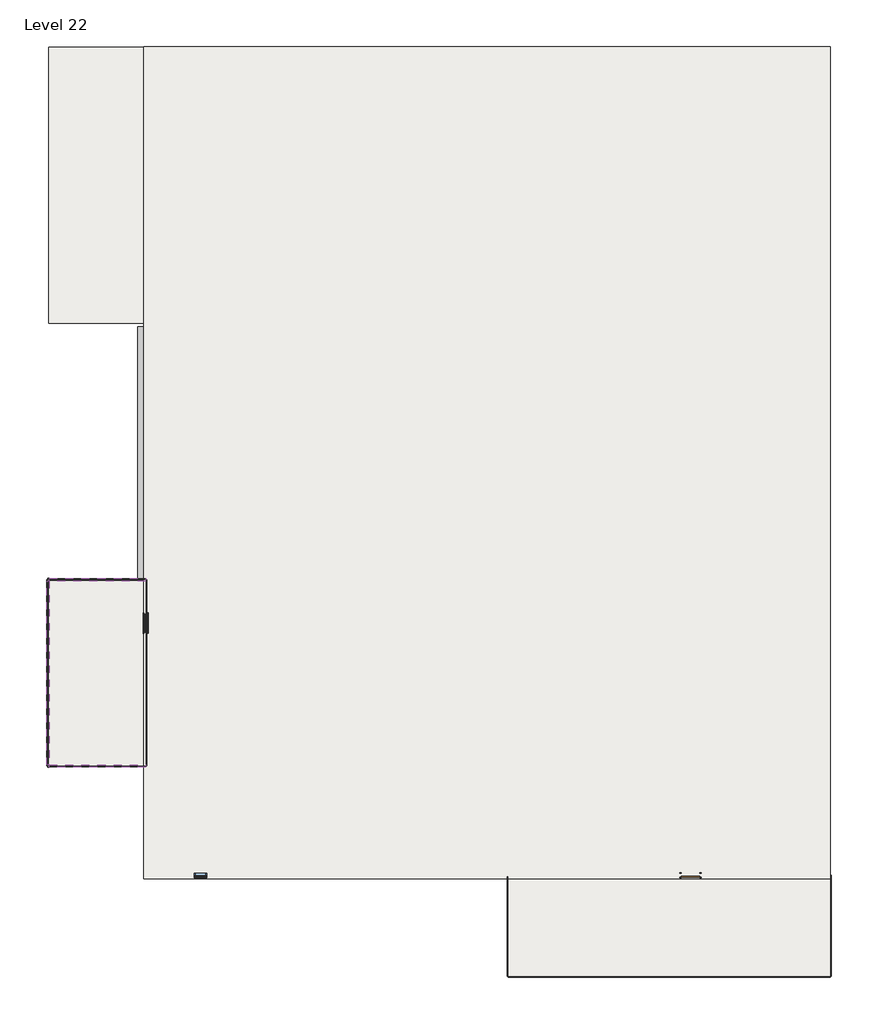
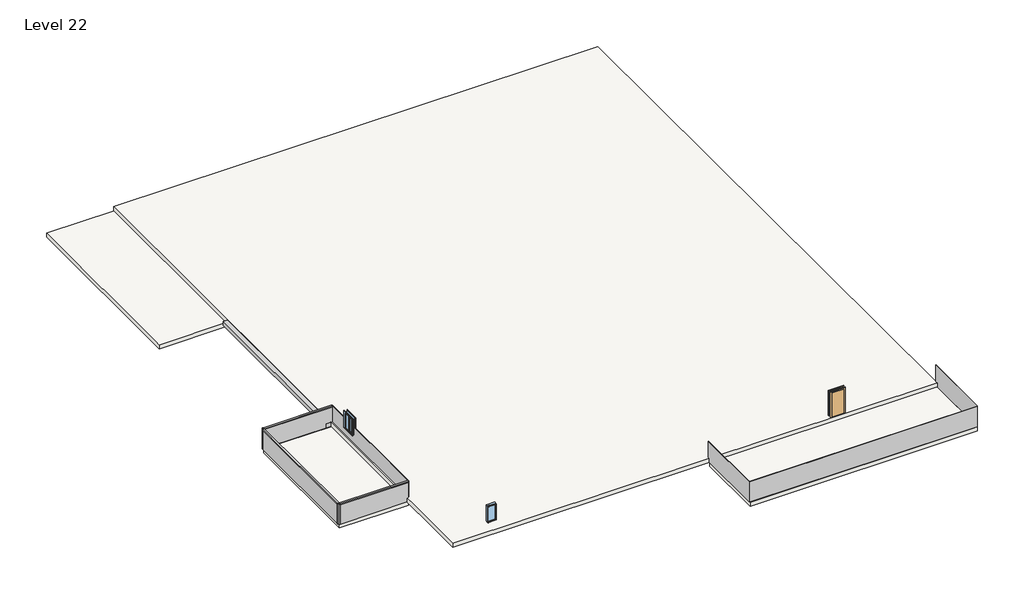
# One storey: 7 members, 7 plates, 4 slabs, 2 windows, 1 door, 1 proxy.
"""IFC4 building model written with IfcOpenShell, lengths in millimetres."""

from ifc_helpers import new_model, si_unit, frame, origin, place, context, project, spatial, polyline, outline, extrude, transform, mapped, element, save
from components import generic_models_7_generic_models_7_7f11944a, door_719f80de, member_4491d118, member_e63cd10b, member_1c0fec03, system_panel_glazed_dbf8c7ac, system_panel_glazed_9f3cc7a8, system_panel_glazed_aa9a1819, system_panel_glazed_da9a879b, system_panel_glazed_ba9ccfd0, system_panel_glazed_4de2f835, window_78885257, window_54100e87

model = new_model("IFC4")

# Units and contexts
model_context = context("Model", 3, world=origin())
ifc_project = project(units=[si_unit("LENGTHUNIT", "METRE", prefix="MILLI")], contexts=[model_context])

# Site, building, storey
site = spatial("IfcSite", under=ifc_project)
building = spatial("IfcBuilding", under=site)
storey = spatial("IfcBuildingStorey", under=building, Name="Level 22", Elevation=36271.2)

# Proxy
placement = place(None, origin())
generic_models_7_generic_models_7_shape = generic_models_7_generic_models_7_7f11944a(model_context)
element("IfcBuildingElementProxy", 1, Name="Generic Models 7 : Generic Models 7", ObjectType="Generic Models 7 : Generic Models 7", at=placement, inside=storey, context=model_context, shape_type="MappedRepresentation", body=[
    mapped(generic_models_7_generic_models_7_shape, transform((0.0, 0.0, 0.0), x_axis=(1.0, 0.0, 0.0), y_axis=(0.0, 1.0, 0.0), z_axis=(0.0, 0.0, 1.0))),
])

# Door
door_shape = door_719f80de(model_context)
element("IfcDoor", 2, ObjectType="Single-Flush : 36\" x 84\"", at=placement, inside=storey, context=model_context, shape_type="MappedRepresentation", body=[
    mapped(door_shape, transform((12155.361926, -20744.1985361, 36271.2), x_axis=(1.0, 0.0, 0.0), y_axis=(0.0, 1.0, 0.0), z_axis=(0.0, 0.0, 1.0))),
])

# Members
member_shape = member_4491d118(model_context)
element("IfcMember", 3, ObjectType="Rectangular Mullion : 2.5\" x 5\" rectangular", at=placement, inside=storey, context=model_context, shape_type="MappedRepresentation", body=[
    mapped(member_shape, transform((-20096.288074, -15263.2213044, 36271.2), x_axis=(-1.0, 0.0, 0.0), y_axis=(0.0, 1.0, 0.0), z_axis=(0.0, 0.0, -1.0))),
])
element("IfcMember", 4, ObjectType="Rectangular Mullion : 2.5\" x 5\" rectangular", at=placement, inside=storey, context=model_context, shape_type="MappedRepresentation", body=[
    mapped(member_shape, transform((-20096.288074, -5922.3713044, 36271.2), x_axis=(0.0, 1.0, 0.0), y_axis=(1.0, 0.0, 0.0), z_axis=(0.0, 0.0, -1.0))),
])
element("IfcMember", 5, ObjectType="Rectangular Mullion : 2.5\" x 5\" rectangular", at=placement, inside=storey, context=model_context, shape_type="MappedRepresentation", body=[
    mapped(member_shape, transform((-20096.288074, -15263.2213044, 37795.2), x_axis=(0.0, -1.0, 0.0), y_axis=(1.0, 0.0, 0.0), z_axis=(0.0, 0.0, 1.0))),
])
element("IfcMember", 6, ObjectType="Rectangular Mullion : 2.5\" x 5\" rectangular", at=placement, inside=storey, context=model_context, shape_type="MappedRepresentation", body=[
    mapped(member_shape, transform((-20096.288074, -5922.3713044, 37795.2), x_axis=(-1.0, 0.0, 0.0), y_axis=(0.0, -1.0, 0.0), z_axis=(0.0, 0.0, 1.0))),
])
member_2_shape = member_e63cd10b(model_context)
element("IfcMember", 7, ObjectType="Rectangular Mullion : 2.5\" x 5\" rectangular", at=placement, inside=storey, context=model_context, shape_type="MappedRepresentation", body=[
    mapped(member_2_shape, transform((-15175.038074, -5922.3713044, 37795.2), x_axis=(0.0, 0.0, 1.0), y_axis=(0.0, -1.0, 0.0), z_axis=(1.0, 0.0, 0.0))),
])
element("IfcMember", 8, ObjectType="Rectangular Mullion : 2.5\" x 5\" rectangular", at=placement, inside=storey, context=model_context, shape_type="MappedRepresentation", body=[
    mapped(member_2_shape, transform((-20032.788074, -15263.2213044, 37795.2), x_axis=(0.0, 0.0, 1.0), y_axis=(0.0, 1.0, 0.0), z_axis=(-1.0, 0.0, 0.0))),
])
member_3_shape = member_1c0fec03(model_context)
element("IfcMember", 9, ObjectType="Rectangular Mullion : 2.5\" x 5\" rectangular", at=placement, inside=storey, context=model_context, shape_type="MappedRepresentation", body=[
    mapped(member_3_shape, transform((-20096.288074, -5985.8713044, 37795.2), x_axis=(0.0, 0.0, 1.0), y_axis=(1.0, 0.0, 0.0), z_axis=(0.0, 1.0, 0.0))),
])

# Plates
system_panel_glazed_shape = system_panel_glazed_dbf8c7ac(model_context)
element("IfcPlate", 10, ObjectType="System Panel : Glazed", at=placement, inside=storey, context=model_context, shape_type="MappedRepresentation", body=[
    mapped(system_panel_glazed_shape, transform((11088.561926, -25828.3670305, 36271.2), x_axis=(-1.0, 0.0, 0.0), y_axis=(0.0, -1.0, 0.0), z_axis=(0.0, 0.0, 1.0))),
])
system_panel_glazed_2_shape = system_panel_glazed_9f3cc7a8(model_context)
element("IfcPlate", 11, ObjectType="System Panel : Glazed", at=placement, inside=storey, context=model_context, shape_type="MappedRepresentation", body=[
    mapped(system_panel_glazed_2_shape, transform((19165.761926, -23286.2827833, 36271.2), x_axis=(0.0, -1.0, 0.0), y_axis=(1.0, 0.0, 0.0), z_axis=(0.0, 0.0, 1.0))),
])
system_panel_glazed_3_shape = system_panel_glazed_aa9a1819(model_context)
element("IfcPlate", 12, ObjectType="System Panel : Glazed", at=placement, inside=storey, context=model_context, shape_type="MappedRepresentation", body=[
    mapped(system_panel_glazed_3_shape, transform((3011.361926, -23326.2903055, 36271.2), x_axis=(0.0, 1.0, 0.0), y_axis=(-1.0, 0.0, 0.0), z_axis=(0.0, 0.0, 1.0))),
])
system_panel_glazed_4_shape = system_panel_glazed_da9a879b(model_context)
element("IfcPlate", 13, ObjectType="System Panel : Glazed", at=placement, inside=storey, context=model_context, shape_type="MappedRepresentation", body=[
    mapped(system_panel_glazed_4_shape, transform((-15175.038074, -10592.7963044, 36271.2), x_axis=(0.0, -1.0, 0.0), y_axis=(1.0, 0.0, 0.0), z_axis=(0.0, 0.0, 1.0))),
])
system_panel_glazed_5_shape = system_panel_glazed_ba9ccfd0(model_context)
element("IfcPlate", 14, ObjectType="System Panel : Glazed", at=placement, inside=storey, context=model_context, shape_type="MappedRepresentation", body=[
    mapped(system_panel_glazed_5_shape, transform((-17603.913074, -5922.3713044, 36271.2), x_axis=(1.0, 0.0, 0.0), y_axis=(0.0, 1.0, 0.0), z_axis=(0.0, 0.0, 1.0))),
])
element("IfcPlate", 15, ObjectType="System Panel : Glazed", at=placement, inside=storey, context=model_context, shape_type="MappedRepresentation", body=[
    mapped(system_panel_glazed_5_shape, transform((-17603.913074, -15263.2213044, 36271.2), x_axis=(-1.0, 0.0, 0.0), y_axis=(0.0, -1.0, 0.0), z_axis=(0.0, 0.0, 1.0))),
])
system_panel_glazed_6_shape = system_panel_glazed_4de2f835(model_context)
element("IfcPlate", 16, ObjectType="System Panel : Glazed", at=placement, inside=storey, context=model_context, shape_type="MappedRepresentation", body=[
    mapped(system_panel_glazed_6_shape, transform((-20096.288074, -10592.7963044, 36271.2), x_axis=(0.0, 1.0, 0.0), y_axis=(-1.0, 0.0, 0.0), z_axis=(0.0, 0.0, 1.0))),
])

# Slabs
element("IfcSlab", 17, ObjectType="Generic - 12\"", at=placement, inside=storey, context=model_context, shape_type="SweptSolid", body=[
    extrude(outline(polyline([(19165.761926, 20833.4253594), (19165.761926, -20924.1746406), (-15276.638074, -20924.1746406), (-15276.638074, 20833.4253594), (19165.761926, 20833.4253594)])), frame((0.0, 0.0, 36258.4195447), z_axis=(0.0, 0.0, 1.0), x_axis=(1.0, 0.0, 0.0)), (0.0, 0.0, 1.0), 304.8),
])
element("IfcSlab", 18, ObjectType="Generic - 12\"", at=placement, inside=storey, context=model_context, shape_type="SweptSolid", body=[
    extrude(outline(polyline([(19165.761926, -20914.1789604), (19165.761926, -25879.1670305), (3011.361926, -25879.1670305), (3011.361926, -20914.1789604), (19165.761926, -20914.1789604)])), frame((0.0, 0.0, 35966.4), z_axis=(0.0, 0.0, 1.0), x_axis=(1.0, 0.0, 0.0)), (0.0, 0.0, 1.0), 304.8),
])
element("IfcSlab", 19, ObjectType="Generic - 12\"", at=placement, inside=storey, context=model_context, shape_type="SweptSolid", body=[
    extrude(outline(polyline([(-20051.838074, -15263.2213044), (-20051.838074, -5966.8213044), (-15175.038074, -5966.8213044), (-15175.038074, -15263.2213044), (-20051.838074, -15263.2213044)])), frame((0.0, 0.0, 35966.4), z_axis=(0.0, 0.0, 1.0), x_axis=(1.0, 0.0, 0.0)), (0.0, 0.0, 1.0), 304.8),
])
element("IfcSlab", 20, ObjectType="Generic - 12\"", at=placement, inside=storey, context=model_context, shape_type="SweptSolid", body=[
    extrude(outline(polyline([(-20051.838074, 20810.2014639), (-15175.038074, 20810.2014639), (-15175.038074, 6941.8014639), (-20051.838074, 6941.8014639), (-20051.838074, 20810.2014639)])), frame((0.0, 0.0, 35966.4), z_axis=(0.0, 0.0, 1.0), x_axis=(1.0, 0.0, 0.0)), (0.0, 0.0, 1.0), 304.8),
])

# Windows
window_shape = window_78885257(model_context)
element("IfcWindow", 21, ObjectType="Instance - Fixed : 24\" x 48\"", at=placement, inside=storey, context=model_context, shape_type="MappedRepresentation", body=[
    mapped(window_shape, transform((-12469.938074, -20744.1985361, 36271.2), x_axis=(-1.0, 0.0, 0.0), y_axis=(0.0, -1.0, 0.0), z_axis=(0.0, 0.0, 1.0))),
])
window_2_shape = window_54100e87(model_context)
element("IfcWindow", 22, ObjectType="Slider with Trim : 36\" x 48\"", at=placement, inside=storey, context=model_context, shape_type="MappedRepresentation", body=[
    mapped(window_2_shape, transform((-15175.038074, -8100.4213044, 36271.2), x_axis=(0.0, 1.0, 0.0), y_axis=(-1.0, 0.0, 0.0), z_axis=(0.0, 0.0, 1.0))),
])

save(model, "model.ifc")

# Revit data of these elements
# Type "Single-Flush : 36\" x 84\""
#   Type Mark = "1"
#   Construction Type Id = "MDOOR"
#   Assembly Code = "C1020"
#   Analytic Construction = "Metal"
#   Thickness = 0' - 2"
#   Heat Transfer Coefficient (U) = 0.651978 BTU/(h·ft²·°F)
#   Height = 7' - 0"
#   Trim Projection Ext = 0' - 1"
#   Trim Projection Int = 0' - 1"
#   Trim Width = 0' - 3"
#   Width = 3' - 0"
#   Define Thermal Properties by = 1
#   Door Material = Door - Panel
#   Frame Material = Door - Frame
#   Visual Light Transmittance = 0
#   Solar Heat Gain Coefficient = 0
#   Function = (empty or 0)
#   Wall Closure = (empty or 0)
# Type "Rectangular Mullion : 2.5\" x 5\" rectangular"
#   built-in parameter 1007304 = 0.416667 (stored number, unit not read)
#   built-in parameter 1007301 = 0.104167 (stored number, unit not read)
#   built-in parameter 1007300 = 0.104167 (stored number, unit not read)
# Type "System Panel : Glazed"
#   Construction Type Id = "GSP4R"
#   Analytic Construction = "1/8 in Pilkington single glazing"
#   Visual Light Transmittance = 0.9
#   Solar Heat Gain Coefficient = 0.86
#   Heat Transfer Coefficient (U) = 1.18115 BTU/(h·ft²·°F)
# Type "Generic - 12\""
#   Assembly Code = "B1010"
#   Function = 0
#   Layers, outside or top first: 1' - 0" no material (function 1)
# Type "Instance - Fixed : 24\" x 48\""
#   Type Mark = "19"
#   Construction Type Id = "GSP4R"
#   Assembly Code = "B2020100"
#   Analytic Construction = "1/8 in Pilkington single glazing"
#   Visual Light Transmittance = 0.9
#   Thermal Resistance (R) = 0.8466 (h·ft²·°F)/BTU
#   Solar Heat Gain Coefficient = 0.86
#   Heat Transfer Coefficient (U) = 1.1812 BTU/(h·ft²·°F)
#   Height [instance default] = 4' - 0"
#   Default Sill Height = 3' - 0"
#   Width [instance default] = 2' - 0"
#   Window Inset = 0' - 0 3/4"
#   Define Thermal Properties by = 1
#   Glass Pane Material = Glass
#   Sash Material = Sash
#   Wall Closure = (empty or 0)
# Type "Slider with Trim : 36\" x 48\""
#   Type Mark = "22"
#   Construction Type Id = "GSP4R"
#   Assembly Code = "B2020100"
#   Analytic Construction = "1/8 in Pilkington single glazing"
#   Visual Light Transmittance = 0.9
#   Solar Heat Gain Coefficient = 0.78
#   Heat Transfer Coefficient (U) = 0.6496 BTU/(h·ft²·°F)
#   Height = 4' - 0"
#   Default Sill Height = 3' - 0"
#   Trim Projection - Ext. = 0' - 0 3/4"
#   Trim Projection - Int. = 0' - 0 3/4"
#   Trim Width - Exterior = 0' - 3 1/2"
#   Trim Width - Interior = 0' - 3 1/2"
#   Width = 3' - 0"
#   Window Inset = 0' - 0 3/4"
#   Define Thermal Properties by = 1
#   Glass Pane Material = Glass
#   Sash Material = Sash
#   Trim Exterior Material = Trim
#   Trim Interior Material = Trim
#   Wall Closure = (empty or 0)
# Element 1 (IfcBuildingElementProxy, "Generic Models 7 : Generic Models 7")
#   Phase Created = New Construction
# Element 2 (IfcDoor, "Single-Flush : 36\" x 84\"")
#   Phase Created = New Construction
#   Materials on its faces: "Door - Frame", "Door - Panel"
# Elements 3, 4, 5, 6, 7, 8, 9 (IfcMember, "Rectangular Mullion : 2.5\" x 5\" rectangular")
#   Phase Created = New Construction
#   Materials on its faces: "Aluminum"
# Elements 10, 11, 12, 13, 14, 15, 16 (IfcPlate, "System Panel : Glazed")
#   Phase Created = New Construction
#   Materials on its faces: "Glass"
# Element 17 (IfcSlab, "Generic - 12\"")
#   Height Offset From Level = 0' - 11.49683"
#   Phase Created = New Construction
#   Materials on its faces: "Default Floor"
# Element 18 (IfcSlab, "Generic - 12\"")
#   Height Offset From Level = 0' - 0"
#   Phase Created = New Construction
#   Materials on its faces: "Default Floor"
# Elements 19, 20 (IfcSlab, "Generic - 12\"")
#   built-in parameter 1001955 = 3.14159 (stored number, unit not read)
#   Height Offset From Level = 0' - 0"
#   Phase Created = New Construction
#   Materials on its faces: "Default Floor"
# Element 21 (IfcWindow, "Instance - Fixed : 24\" x 48\"")
#   Mark = "12"
#   Width = 2' - 0"
#   Height = 4' - 0"
#   Phase Created = New Construction
#   Materials on its faces: "Sash", "Glass"
# Element 22 (IfcWindow, "Slider with Trim : 36\" x 48\"")
#   Mark = "34"
#   Phase Created = New Construction
#   Materials on its faces: "Sash", "Trim", "Glass"
# Materials
#   "Door - Panel": class "Wood", colour RGB 210 159 95, transparency 0
#   "Door - Frame": colour RGB 118 70 51, transparency 0
#   "Glass": class "Glass", colour RGB 0 128 192, transparency 0.75, Description = "Soda Lime Glass", Cost = 0
#   "Sash": class "Wood", colour RGB 224 178 126, transparency 0
#   "Trim": class "Wood", colour RGB 224 178 126, transparency 0
#   "Aluminum": class "Metal", colour RGB 247 247 247, transparency 0, Description = "Aluminum 6061", Cost = 0
#   "Default Floor": colour RGB 128 128 128, transparency 0
